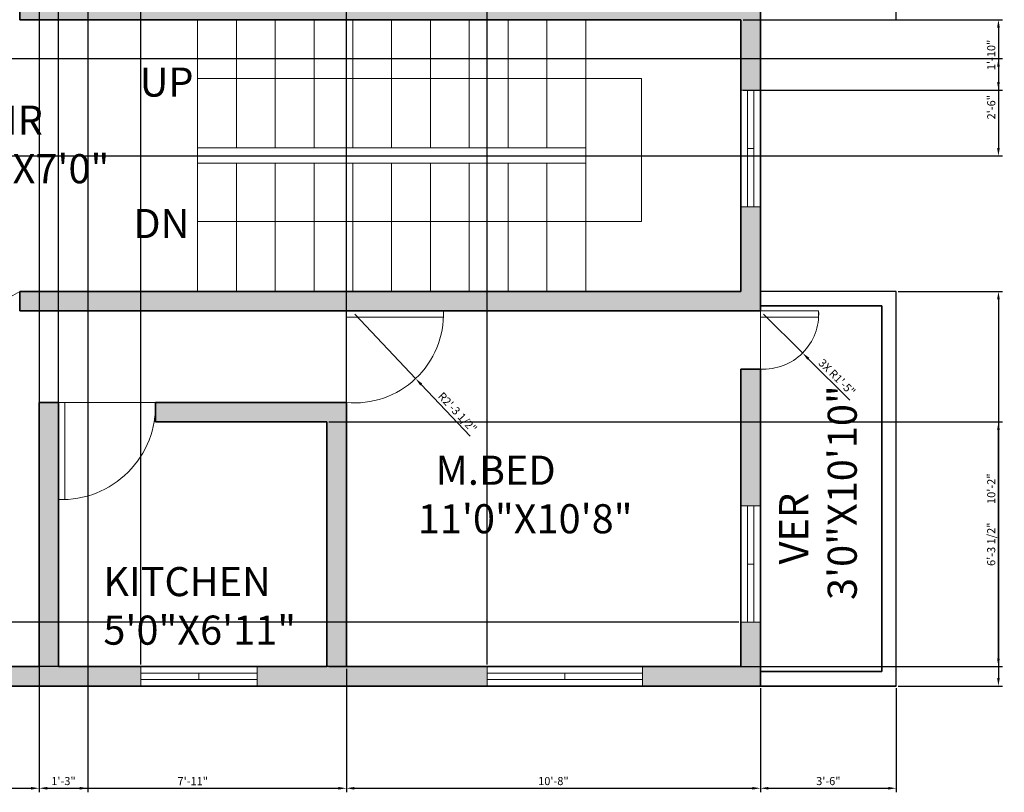
# Model space of a CAD drawing. Units: inches. Extents: x 5145 to 5807, y 9597 to 10060.
# Tile 2 of 3: x 5502 to 5807, y 9597 to 9836. Entities that reach past the tile are written whole.
import ezdxf

# ---------------------------------------------------------------- set-up
doc = ezdxf.new("R2010")
doc.units = ezdxf.units.IN
for name, color, linetype, lineweight in [('A-ANNO-DIMS', 7, 'Continuous', 18), ('A-AREA-IDEN', 7, 'Continuous', 18), ('A-GLAZ', 140, 'Continuous', 18), ('A-WALL', 7, 'Continuous', 35)]:
    doc.layers.add(name, color=color, linetype=linetype, lineweight=lineweight)
for name, color, linetype, lineweight, true_color in [('A-ANNO-SYMB', 244, 'Continuous', 18, 0x991b1e), ('A-ANNO-TEXT', 244, 'Continuous', 18, 0x991b1e), ('A-DOOR', 2, 'Continuous', 18, 0xf1eb1f), ('A-FLOR-STRS', 30, 'Continuous', 18, 0xf26722), ('A-WALL-PATT', 159, 'Continuous', 13, 0x22346e), ('A-WALL-PRPT', 61, 'Continuous', 25, 0xedee99)]:
    doc.layers.add(name, color=color, linetype=linetype, lineweight=lineweight, true_color=true_color)
doc.styles.get("Standard").update_dxf_attribs({"font": 'arial.ttf'})
doc.dimstyles.new('ISO-25', dxfattribs={"dimtxt": 2.5, "dimasz": 2.5, "dimexe": 1.25, "dimexo": 0.625, "dimtad": 1, "dimlunit": 3, "dimtxsty": 'Standard', "dimcen": 2.5, "dimadec": 0, "dimazin": 0, "dimtfac": 1, "dimtmove": 0, "dimatfit": 3, "dimfxl": 1, "dimarcsym": 0})

# ---------------------------------------------------------------- blocks, each defined once
blk = doc.blocks.new('WIN-36IN')
for p, q in [((0, 6), (0, 0)), ((0, 6), (36, 6)), ((0, 4), (36, 4)), ((18, 2), (18, 4)), ((36, 0), (36, 6)), ((0, 2), (36, 2)), ((36, 0), (0, 0))]:
    blk.add_line(p, q)
blk = doc.blocks.new('WIN-48IN')
for p, q in [((6, 48), (0, 48)), ((0, 48), (0, 0)), ((2, 0), (2, 48)), ((4, 0), (4, 48)), ((6, 0), (6, 48)), ((4, 24), (2, 24)), ((0, 0), (6, 0))]:
    blk.add_line(p, q)
blk = doc.blocks.new('DOOR-SWING-18IN')
for p, q in [((0.03, 18.03), (18.03, 18.03)), ((16.03, 0.03), (16.03, 18.03)), ((16.03, 18.03), (18.03, 18.03)), ((18.03, 18.03), (18.03, 0.03)), ((18.03, 0.03), (16.03, 0.03))]:
    blk.add_line(p, q)
blk.add_arc((17.03, 17.03), 17.03, 176.6335, 273.3665)
blk = doc.blocks.new('DOOR-SWING-30IN')
for p, q in [((0, 0), (0, 30)), ((0, 30), (2, 30)), ((2, 30), (2, 0)), ((2, 0), (0, 0)), ((0, 0), (30, 0))]:
    blk.add_line(p, q)
blk.add_arc((1, 1), 29.02, 358.0251, 91.9749)
blk = doc.blocks.new('*D23')
at = {"layer": 'A-ANNO-DIMS', "color": 0, "lineweight": -2, "transparency": 16777216}
for p, q in [((5329.12, 9635.64), (5329.12, 9597.42)), ((5508.12, 9635.64), (5508.12, 9597.42)), ((5331.62, 9598.67), (5505.62, 9598.67))]:
    blk.add_line(p, q, dxfattribs=at)
at = {"layer": 'A-ANNO-DIMS', "color": 0, "transparency": 16777216}
for points in [[(5331.62, 9599.08), (5331.62, 9598.25), (5329.12, 9598.67)], [(5505.62, 9599.08), (5505.62, 9598.25), (5508.12, 9598.67)]]:
    blk.add_solid(points, dxfattribs=at)
at = {"layer": 'Defpoints', "color": 0, "transparency": 16777216}
for p in [(5329.12, 9636.27), (5508.12, 9636.27), (5508.12, 9598.67)]:
    blk.add_point(p, dxfattribs=at)
at = {"layer": 'A-ANNO-DIMS', "color": 0, "transparency": 16777216, "insert": (5418.62, 9600.55), "char_height": 2.5, "attachment_point": 5}
blk.add_mtext('14\'-11"', dxfattribs=at)
blk = doc.blocks.new('*D24')
at = {"layer": 'A-ANNO-DIMS', "color": 0, "lineweight": -2, "transparency": 16777216}
for p, q in [((5508.12, 9635.64), (5508.12, 9597.42)), ((5603.12, 9635.64), (5603.12, 9597.42)), ((5510.62, 9598.67), (5600.62, 9598.67))]:
    blk.add_line(p, q, dxfattribs=at)
at = {"layer": 'A-ANNO-DIMS', "color": 0, "transparency": 16777216}
for points in [[(5510.62, 9599.08), (5510.62, 9598.25), (5508.12, 9598.67)], [(5600.62, 9599.08), (5600.62, 9598.25), (5603.12, 9598.67)]]:
    blk.add_solid(points, dxfattribs=at)
at = {"layer": 'Defpoints', "color": 0, "transparency": 16777216}
for p in [(5508.12, 9636.27), (5603.12, 9636.27), (5603.12, 9598.67)]:
    blk.add_point(p, dxfattribs=at)
at = {"layer": 'A-ANNO-DIMS', "color": 0, "transparency": 16777216, "insert": (5555.62, 9600.55), "char_height": 2.5, "attachment_point": 5}
blk.add_mtext('7\'-11"', dxfattribs=at)
blk = doc.blocks.new('*D25')
at = {"layer": 'A-ANNO-DIMS', "color": 0, "lineweight": -2, "transparency": 16777216}
for p, q in [((5603.12, 9635.64), (5603.12, 9597.42)), ((5731.12, 9629.64), (5731.12, 9597.42)), ((5605.62, 9598.67), (5728.62, 9598.67))]:
    blk.add_line(p, q, dxfattribs=at)
at = {"layer": 'A-ANNO-DIMS', "color": 0, "transparency": 16777216}
for points in [[(5605.62, 9599.08), (5605.62, 9598.25), (5603.12, 9598.67)], [(5728.62, 9599.08), (5728.62, 9598.25), (5731.12, 9598.67)]]:
    blk.add_solid(points, dxfattribs=at)
at = {"layer": 'Defpoints', "color": 0, "transparency": 16777216}
for p in [(5603.12, 9636.27), (5731.12, 9630.27), (5731.12, 9598.67)]:
    blk.add_point(p, dxfattribs=at)
at = {"layer": 'A-ANNO-DIMS', "color": 0, "transparency": 16777216, "insert": (5667.12, 9600.57), "char_height": 2.5, "attachment_point": 5}
blk.add_mtext('10\'-8"', dxfattribs=at)
blk = doc.blocks.new('*D26')
at = {"layer": 'A-ANNO-DIMS', "color": 0, "lineweight": -2, "transparency": 16777216}
for p, q in [((5731.12, 9629.64), (5731.12, 9597.42)), ((5773.12, 9629.64), (5773.12, 9597.42)), ((5733.62, 9598.67), (5770.62, 9598.67))]:
    blk.add_line(p, q, dxfattribs=at)
at = {"layer": 'A-ANNO-DIMS', "color": 0, "transparency": 16777216}
for points in [[(5733.62, 9599.08), (5733.62, 9598.25), (5731.12, 9598.67)], [(5770.62, 9599.08), (5770.62, 9598.25), (5773.12, 9598.67)]]:
    blk.add_solid(points, dxfattribs=at)
at = {"layer": 'Defpoints', "color": 0, "transparency": 16777216}
for p in [(5731.12, 9630.27), (5773.12, 9630.27), (5773.12, 9598.67)]:
    blk.add_point(p, dxfattribs=at)
at = {"layer": 'A-ANNO-DIMS', "color": 0, "transparency": 16777216, "insert": (5752.12, 9600.57), "char_height": 2.5, "attachment_point": 5}
blk.add_mtext('3\'-6"', dxfattribs=at)
blk = doc.blocks.new('*D28')
at = {"layer": 'A-ANNO-DIMS', "color": 0, "lineweight": -2, "transparency": 16777216}
for p, q in [((5773.74, 9752.27), (5805.97, 9752.27)), ((5804.72, 9749.77), (5804.72, 9632.77)), ((5773.74, 9630.27), (5805.97, 9630.27))]:
    blk.add_line(p, q, dxfattribs=at)
at = {"layer": 'A-ANNO-DIMS', "color": 0, "transparency": 16777216}
for points in [[(5804.3, 9749.77), (5805.13, 9749.77), (5804.72, 9752.27)], [(5804.3, 9632.77), (5805.13, 9632.77), (5804.72, 9630.27)]]:
    blk.add_solid(points, dxfattribs=at)
at = {"layer": 'Defpoints', "color": 0, "transparency": 16777216}
for p in [(5773.12, 9752.27), (5773.12, 9630.27), (5804.72, 9630.27)]:
    blk.add_point(p, dxfattribs=at)
at = {"layer": 'A-ANNO-DIMS', "color": 0, "transparency": 16777216, "insert": (5802.81, 9691.27), "char_height": 2.5, "attachment_point": 5, "rotation": 90}
blk.add_mtext('10\'-2"', dxfattribs=at)
blk = doc.blocks.new('*D30')
at = {"layer": 'A-ANNO-DIMS', "color": 0, "lineweight": -2, "transparency": 16777216}
for p, q in [((5597.74, 9711.93), (5805.97, 9711.93)), ((5804.72, 9638.77), (5804.72, 9709.43)), ((5597.74, 9636.27), (5805.97, 9636.27))]:
    blk.add_line(p, q, dxfattribs=at)
at = {"layer": 'A-ANNO-DIMS', "color": 0, "transparency": 16777216}
for points in [[(5804.3, 9709.43), (5805.13, 9709.43), (5804.72, 9711.93)], [(5804.3, 9638.77), (5805.13, 9638.77), (5804.72, 9636.27)]]:
    blk.add_solid(points, dxfattribs=at)
at = {"layer": 'Defpoints', "color": 0, "transparency": 16777216}
for p in [(5597.12, 9711.93), (5804.72, 9711.93), (5597.12, 9636.27)]:
    blk.add_point(p, dxfattribs=at)
at = {"layer": 'A-ANNO-DIMS', "color": 0, "transparency": 16777216, "insert": (5802.8, 9674.1), "char_height": 2.5, "attachment_point": 5, "rotation": 90}
blk.add_mtext('6\'-3 1/2"', dxfattribs=at)
blk = doc.blocks.new('*D37')
at = {"layer": 'A-ANNO-DIMS', "color": 0, "lineweight": -2, "transparency": 16777216}
for p, q in [((5508.12, 10015.64), (5508.12, 9597.42)), ((5523.2, 10015.64), (5523.2, 9597.42)), ((5510.62, 9598.67), (5520.7, 9598.67))]:
    blk.add_line(p, q, dxfattribs=at)
at = {"layer": 'A-ANNO-DIMS', "color": 0, "transparency": 16777216}
for points in [[(5510.62, 9599.08), (5510.62, 9598.25), (5508.12, 9598.67)], [(5520.7, 9599.08), (5520.7, 9598.25), (5523.2, 9598.67)]]:
    blk.add_solid(points, dxfattribs=at)
at = {"layer": 'Defpoints', "color": 0, "transparency": 16777216}
for p in [(5508.12, 10016.27), (5523.2, 10016.27), (5523.2, 9598.67)]:
    blk.add_point(p, dxfattribs=at)
at = {"layer": 'A-ANNO-DIMS', "color": 0, "transparency": 16777216, "insert": (5515.66, 9600.57), "char_height": 2.5, "attachment_point": 5}
blk.add_mtext('1\'-3"', dxfattribs=at)
blk = doc.blocks.new('*D43')
at = {"layer": 'A-ANNO-DIMS', "color": 0, "lineweight": -2, "transparency": 16777216}
for p, q in [((5514.12, 9636.89), (5514.12, 10055.12)), ((5539.54, 9636.89), (5539.54, 10055.12)), ((5516.62, 10053.87), (5537.04, 10053.87))]:
    blk.add_line(p, q, dxfattribs=at)
at = {"layer": 'A-ANNO-DIMS', "color": 0, "transparency": 16777216}
for points in [[(5516.62, 10054.28), (5516.62, 10053.45), (5514.12, 10053.87)], [(5537.04, 10054.28), (5537.04, 10053.45), (5539.54, 10053.87)]]:
    blk.add_solid(points, dxfattribs=at)
at = {"layer": 'Defpoints', "color": 0, "transparency": 16777216}
for p in [(5539.54, 10053.87), (5514.12, 9636.27), (5539.54, 9636.27)]:
    blk.add_point(p, dxfattribs=at)
at = {"layer": 'A-ANNO-DIMS', "color": 0, "transparency": 16777216, "insert": (5526.83, 10055.79), "char_height": 2.5, "attachment_point": 5}
blk.add_mtext('2\'-1 1/2"', dxfattribs=at)
blk = doc.blocks.new('*D44')
at = {"layer": 'A-ANNO-DIMS', "color": 0, "lineweight": -2, "transparency": 16777216}
for p, q in [((5603.12, 9636.89), (5603.12, 10055.12)), ((5646.69, 9636.89), (5646.69, 10055.12)), ((5605.62, 10053.87), (5644.19, 10053.87))]:
    blk.add_line(p, q, dxfattribs=at)
at = {"layer": 'A-ANNO-DIMS', "color": 0, "transparency": 16777216}
for points in [[(5605.62, 10054.28), (5605.62, 10053.45), (5603.12, 10053.87)], [(5644.19, 10054.28), (5644.19, 10053.45), (5646.69, 10053.87)]]:
    blk.add_solid(points, dxfattribs=at)
at = {"layer": 'Defpoints', "color": 0, "transparency": 16777216}
for p in [(5646.69, 10053.87), (5603.12, 9636.27), (5646.69, 9636.27)]:
    blk.add_point(p, dxfattribs=at)
at = {"layer": 'A-ANNO-DIMS', "color": 0, "transparency": 16777216, "insert": (5624.91, 10055.79), "char_height": 2.5, "attachment_point": 5}
blk.add_mtext('3\'-7 1/2"', dxfattribs=at)
blk = doc.blocks.new('*D46')
at = {"layer": 'A-ANNO-DIMS', "color": 0, "lineweight": -2, "transparency": 16777216}
for p, q in [((5188.74, 9824.27), (5805.97, 9824.27)), ((5804.72, 9821.77), (5804.72, 9796.64)), ((5188.74, 9794.14), (5805.97, 9794.14))]:
    blk.add_line(p, q, dxfattribs=at)
at = {"layer": 'A-ANNO-DIMS', "color": 0, "transparency": 16777216}
for points in [[(5804.3, 9821.77), (5805.13, 9821.77), (5804.72, 9824.27)], [(5804.3, 9796.64), (5805.13, 9796.64), (5804.72, 9794.14)]]:
    blk.add_solid(points, dxfattribs=at)
at = {"layer": 'Defpoints', "color": 0, "transparency": 16777216}
for p in [(5188.12, 9824.27), (5188.12, 9794.14), (5804.72, 9794.14)]:
    blk.add_point(p, dxfattribs=at)
at = {"layer": 'A-ANNO-DIMS', "color": 0, "transparency": 16777216, "insert": (5802.81, 9809.2), "char_height": 2.5, "attachment_point": 5, "rotation": 90}
blk.add_mtext('2\'-6"', dxfattribs=at)
blk = doc.blocks.new('*D48')
at = {"layer": 'A-ANNO-DIMS', "color": 0, "lineweight": -2, "transparency": 16777216}
for p, q in [((5725.74, 9836.27), (5805.97, 9836.27)), ((5804.72, 9833.77), (5804.72, 9816.96)), ((5725.74, 9814.46), (5805.97, 9814.46))]:
    blk.add_line(p, q, dxfattribs=at)
at = {"layer": 'A-ANNO-DIMS', "color": 0, "transparency": 16777216}
for points in [[(5804.3, 9833.77), (5805.13, 9833.77), (5804.72, 9836.27)], [(5804.3, 9816.96), (5805.13, 9816.96), (5804.72, 9814.46)]]:
    blk.add_solid(points, dxfattribs=at)
at = {"layer": 'Defpoints', "color": 0, "transparency": 16777216}
for p in [(5725.12, 9836.27), (5725.12, 9814.46), (5804.72, 9814.46)]:
    blk.add_point(p, dxfattribs=at)
at = {"layer": 'A-ANNO-DIMS', "color": 0, "transparency": 16777216, "insert": (5802.81, 9825.36), "char_height": 2.5, "attachment_point": 5, "rotation": 90}
blk.add_mtext('1\'-10"', dxfattribs=at)
blk = doc.blocks.new('*D49')
at = {"layer": 'A-ANNO-DIMS', "color": 0, "lineweight": -2, "transparency": 16777216}
for p, q in [((5724.49, 9649.99), (5149.27, 9649.99)), ((5150.52, 9638.77), (5150.52, 9647.49)), ((5724.49, 9636.27), (5149.27, 9636.27))]:
    blk.add_line(p, q, dxfattribs=at)
at = {"layer": 'A-ANNO-DIMS', "color": 0, "transparency": 16777216}
for points in [[(5150.1, 9647.49), (5150.93, 9647.49), (5150.52, 9649.99)], [(5150.1, 9638.77), (5150.93, 9638.77), (5150.52, 9636.27)]]:
    blk.add_solid(points, dxfattribs=at)
at = {"layer": 'Defpoints', "color": 0, "transparency": 16777216}
for p in [(5150.52, 9649.99), (5725.12, 9649.99), (5725.12, 9636.27)]:
    blk.add_point(p, dxfattribs=at)
at = {"layer": 'A-ANNO-DIMS', "color": 0, "transparency": 16777216, "insert": (5148.6, 9643.13), "char_height": 2.5, "attachment_point": 5, "rotation": 90}
blk.add_mtext('1\'-1 1/2"', dxfattribs=at)
blk = doc.blocks.new('*D55')
at = {"layer": 'A-ANNO-DIMS', "color": 0, "lineweight": -2, "transparency": 16777216}
for p, q in [((5605.68, 9745.27), (5624.53, 9725.31)), ((5641.38, 9707.47), (5626.25, 9723.49))]:
    blk.add_line(p, q, dxfattribs=at)
at = {"layer": 'A-ANNO-DIMS', "color": 0, "transparency": 16777216}
blk.add_solid([(5626.55, 9723.78), (5625.95, 9723.2), (5624.53, 9725.31)], dxfattribs=at)
at = {"layer": 'Defpoints', "color": 0, "transparency": 16777216}
for p in [(5605.68, 9745.27), (5624.53, 9725.31)]:
    blk.add_point(p, dxfattribs=at)
at = {"layer": 'A-ANNO-DIMS', "color": 0, "transparency": 16777216, "insert": (5637.24, 9714.65), "char_height": 2.5, "attachment_point": 5, "rotation": 313.3682}
blk.add_mtext('R2\'-3 1/2"', dxfattribs=at)
blk = doc.blocks.new('*D58')
at = {"layer": 'A-ANNO-DIMS', "color": 0, "lineweight": -2, "transparency": 16777216}
for p, q in [((5732.12, 9745.27), (5744.16, 9733.23)), ((5758.77, 9718.62), (5745.93, 9731.46))]:
    blk.add_line(p, q, dxfattribs=at)
at = {"layer": 'A-ANNO-DIMS', "color": 0, "transparency": 16777216}
blk.add_solid([(5746.22, 9731.75), (5745.63, 9731.16), (5744.16, 9733.23)], dxfattribs=at)
at = {"layer": 'Defpoints', "color": 0, "transparency": 16777216}
for p in [(5732.12, 9745.27), (5744.16, 9733.23)]:
    blk.add_point(p, dxfattribs=at)
at = {"layer": 'A-ANNO-DIMS', "color": 0, "transparency": 16777216, "insert": (5754.57, 9725.5), "char_height": 2.5, "attachment_point": 5, "rotation": 315.0004}
blk.add_mtext('3X R1\'-5"', dxfattribs=at)

msp = doc.modelspace()

# ---------------------------------------------------------------- hatches: boundary and pattern name
at = {"layer": 'A-WALL-PATT'}
h = msp.add_hatch(color=256, dxfattribs=at)
h.dxf.hatch_style = 1
h.paths.add_polyline_path([(5244.116, 10016.267), (5266.307, 10016.267), (5266.307, 10022.267), (5238.116, 10022.267), (5238.116, 10017.767), (5238.116, 9962.267), (5329.116, 9962.267), (5329.116, 9968.267), (5311.116, 9968.267), (5244.116, 9968.267)])
h.paths.add_polyline_path([(5372.995, 10022.267), (5290.307, 10022.267), (5290.307, 10016.267), (5323.116, 10016.267), (5323.116, 9986.267), (5327.116, 9986.267, -0.0293864), (5329.116, 9986.267), (5329.116, 10016.267), (5372.995, 10016.267)])
h.paths.add_polyline_path([(5523.196, 10022.267), (5432.995, 10022.267), (5432.995, 10016.267), (5502.116, 10016.267), (5502.116, 9878.267), (5508.116, 9878.267), (5508.116, 9908.267), (5508.116, 10016.267), (5523.196, 10016.267)])
h.paths.add_polyline_path([(5623.247, 10022.267), (5559.196, 10022.267), (5559.196, 10016.267), (5591.116, 10016.267), (5591.116, 9884.267), (5538.116, 9884.267), (5538.116, 9880.267, -0.0172363), (5538.116, 9878.267), (5597.116, 9878.267), (5597.116, 10016.267), (5623.247, 10016.267)])
h.paths.add_polyline_path([(5731.116, 10022.267), (5695.247, 10022.267), (5695.247, 10016.267), (5725.116, 10016.267), (5725.116, 9968.267), (5731.116, 9968.267)])
h.paths.add_polyline_path([(5731.116, 9920.267), (5725.116, 9920.267), (5725.116, 9860.267, -0.0293864), (5727.116, 9860.267), (5731.116, 9860.267)])
h.paths.add_polyline_path([(5731.116, 9842.267), (5725.116, 9842.267), (5502.116, 9842.267), (5502.116, 9836.267), (5725.116, 9836.267), (5725.116, 9814.459), (5731.116, 9814.459)])
h.paths.add_polyline_path([(5731.116, 9778.459), (5725.116, 9778.459), (5725.116, 9752.267), (5502.116, 9752.267), (5502.116, 9746.267), (5731.116, 9746.267)])
h.paths.add_polyline_path([(5514.116, 9717.93), (5508.116, 9717.93), (5508.116, 9704.267), (5508.116, 9636.267), (5460.439, 9636.267), (5460.439, 9630.267), (5539.543, 9630.267), (5539.543, 9636.267), (5514.116, 9636.267), (5514.116, 9704.267)])
h.paths.add_polyline_path([(5603.116, 9717.93), (5544.116, 9717.93, -0.0172363), (5544.116, 9715.93), (5544.116, 9711.93), (5597.116, 9711.93), (5597.116, 9636.267), (5575.543, 9636.267), (5575.543, 9630.267), (5646.695, 9630.267), (5646.695, 9636.267), (5603.116, 9636.267), (5603.116, 9704.267)])
h.paths.add_polyline_path([(5731.116, 9649.987), (5725.116, 9649.987), (5725.116, 9636.267), (5694.695, 9636.267), (5694.695, 9630.267), (5731.116, 9630.267)])
h.paths.add_polyline_path([(5731.116, 9728.267), (5725.116, 9728.267), (5725.116, 9685.987), (5731.116, 9685.987)])
h.paths.add_polyline_path([(5400.439, 9636.267), (5329.116, 9636.267), (5329.116, 9662.267, -0.0217289), (5327.116, 9662.267), (5323.116, 9662.267), (5323.116, 9636.267), (5283.616, 9636.267), (5283.616, 9630.267), (5329.116, 9630.267), (5400.439, 9630.267)])
h.paths.add_polyline_path([(5263.165, 9636.267), (5244.116, 9636.267), (5244.116, 9686.267), (5329.116, 9686.267), (5329.116, 9692.267), (5287.116, 9692.267), (5238.116, 9692.267), (5238.116, 9674.267), (5238.116, 9630.267), (5263.165, 9630.267)])
h.paths.add_polyline_path([(5220.116, 9690.267, -0.0293864), (5220.116, 9692.267), (5188.116, 9692.267), (5188.116, 9734.135), (5182.116, 9734.135), (5182.116, 9686.267), (5220.116, 9686.267)])
h.paths.add_polyline_path([(5329.116, 9794.267), (5469.593, 9794.267), (5469.593, 9800.267), (5427.593, 9800.267), (5329.116, 9800.267), (5329.116, 9830.267), (5329.116, 9920.267, -0.0121933), (5327.116, 9920.267), (5323.116, 9920.267), (5323.116, 9830.267), (5188.116, 9830.267), (5188.116, 9865.614), (5182.116, 9865.614), (5182.116, 9794.135), (5188.116, 9794.135), (5188.116, 9824.267), (5323.116, 9824.267), (5323.116, 9734.267), (5327.116, 9734.267, -0.0121933), (5329.116, 9734.267)])

# ---------------------------------------------------------------- linework, layer by layer
at = {"layer": 'A-ANNO-SYMB'}
for p, q in [((5694.376, 9818.125), (5557.116, 9818.125)), ((5694.376, 9773.836), (5694.376, 9818.125)), ((5557.116, 9773.836), (5694.376, 9773.836))]:
    msp.add_line(p, q, dxfattribs=at)
at = {"layer": 'A-DOOR'}
for p, q in [((5603.116, 9746.267), (5633.116, 9746.267)), ((5603.116, 9744.267), (5603.116, 9746.267)), ((5603.116, 9717.93), (5603.116, 9746.267)), ((5633.116, 9744.267), (5603.116, 9744.267)), ((5633.116, 9746.267), (5633.116, 9744.267))]:
    msp.add_line(p, q, dxfattribs=at)
for centre, radius, start, end in [((5476.126, 9793.267), 48.544, 178.81962, 302.37097), ((5605.677, 9745.267), 27.457, 264.64826, 2.08719)]:
    msp.add_arc(centre, radius, start, end, dxfattribs=at)
at = {"layer": 'A-FLOR-STRS'}
for p, q in [((5557.116, 9836.267), (5557.116, 9752.267)), ((5569.116, 9836.267), (5569.116, 9796.667)), ((5581.116, 9836.267), (5581.116, 9796.667)), ((5593.116, 9836.267), (5593.116, 9796.667)), ((5605.116, 9836.267), (5605.116, 9796.667)), ((5617.116, 9836.267), (5617.116, 9796.667)), ((5629.116, 9836.267), (5629.116, 9796.667)), ((5641.116, 9836.267), (5641.116, 9796.667)), ((5653.116, 9836.267), (5653.116, 9796.667)), ((5665.116, 9836.267), (5665.116, 9796.667)), ((5677.116, 9752.267), (5677.116, 9836.267)), ((5677.116, 9836.267), (5677.116, 9752.267)), ((5557.116, 9796.667), (5677.116, 9796.667)), ((5557.116, 9796.667), (5677.116, 9796.667)), ((5557.116, 9791.867), (5677.116, 9791.867)), ((5557.116, 9791.867), (5677.116, 9791.867)), ((5569.116, 9791.867), (5569.116, 9752.267)), ((5581.116, 9791.867), (5581.116, 9752.267)), ((5593.116, 9791.867), (5593.116, 9752.267)), ((5605.116, 9791.867), (5605.116, 9752.267)), ((5617.116, 9791.867), (5617.116, 9752.267)), ((5629.116, 9791.867), (5629.116, 9752.267)), ((5641.116, 9791.867), (5641.116, 9752.267)), ((5653.116, 9791.867), (5653.116, 9752.267)), ((5665.116, 9791.867), (5665.116, 9752.267))]:
    msp.add_line(p, q, dxfattribs=at)
at = {"layer": 'A-GLAZ'}
for p, q in [((5725.116, 9814.459), (5731.116, 9814.459)), ((5731.116, 9778.459), (5731.116, 9814.459)), ((5731.116, 9778.459), (5725.116, 9778.459)), ((5725.116, 9685.987), (5731.116, 9685.987)), ((5731.116, 9649.987), (5731.116, 9685.987)), ((5725.116, 9649.987), (5731.116, 9649.987)), ((5539.543, 9630.267), (5539.543, 9636.267)), ((5575.543, 9636.267), (5575.543, 9630.267)), ((5646.695, 9630.267), (5646.695, 9636.267)), ((5694.695, 9636.267), (5694.695, 9630.267)), ((5539.543, 9630.267), (5575.543, 9630.267)), ((5646.695, 9630.267), (5694.695, 9630.267))]:
    msp.add_line(p, q, dxfattribs=at)
at = {"layer": 'A-WALL'}
for p, q in [((5502.116, 9842.267), (5502.116, 9836.267)), ((5731.116, 9746.267), (5731.116, 9842.267)), ((5502.116, 9836.267), (5725.116, 9836.267)), ((5725.116, 9752.267), (5725.116, 9836.267)), ((5502.116, 9752.267), (5725.116, 9752.267)), ((5502.116, 9752.267), (5502.116, 9746.267)), ((5502.116, 9746.267), (5731.116, 9746.267)), ((5725.116, 9636.267), (5725.116, 9728.267)), ((5725.116, 9728.267), (5731.116, 9728.267)), ((5731.116, 9630.267), (5731.116, 9728.267)), ((5514.116, 9717.93), (5508.116, 9717.93)), ((5508.116, 9717.93), (5508.116, 9704.267)), ((5514.116, 9704.267), (5514.116, 9717.93)), ((5603.116, 9717.93), (5544.116, 9717.93)), ((5544.116, 9711.93), (5544.116, 9717.93)), ((5603.116, 9717.93), (5603.116, 9704.267)), ((5603.116, 9704.267), (5603.116, 9717.93)), ((5597.116, 9711.93), (5544.116, 9711.93)), ((5597.116, 9636.267), (5597.116, 9711.93)), ((5508.116, 9636.267), (5508.116, 9704.267)), ((5514.116, 9636.267), (5514.116, 9704.267)), ((5603.116, 9636.267), (5603.116, 9704.267)), ((5329.116, 9636.267), (5508.116, 9636.267)), ((5514.116, 9636.267), (5597.116, 9636.267)), ((5603.116, 9636.267), (5725.116, 9636.267)), ((5329.116, 9630.267), (5773.116, 9630.267))]:
    msp.add_line(p, q, dxfattribs=at)
at = {"layer": 'A-WALL-PRPT'}
for p, q in [((5773.116, 9836.267), (5773.116, 10022.267)), ((5773.116, 9836.267), (5773.116, 9878.267)), ((5731.116, 9836.267), (5773.116, 9836.267)), ((5731.116, 9836.267), (5773.116, 9836.267)), ((5773.116, 9752.267), (5731.116, 9752.267)), ((5773.116, 9752.267), (5731.116, 9752.267)), ((5773.116, 9746.267), (5773.116, 9752.267)), ((5773.116, 9630.267), (5773.116, 9752.267)), ((5768.616, 9747.767), (5731.116, 9747.767)), ((5731.116, 9747.767), (5768.616, 9747.767)), ((5768.616, 9662.267), (5768.616, 9747.767)), ((5768.616, 9747.767), (5768.616, 9634.767)), ((5773.116, 9662.267), (5773.116, 9746.267)), ((5768.616, 9634.767), (5768.616, 9662.267)), ((5773.116, 9630.267), (5773.116, 9662.267)), ((5731.116, 9634.767), (5768.616, 9634.767)), ((5768.616, 9634.767), (5731.116, 9634.767)), ((5731.116, 9630.267), (5773.116, 9630.267))]:
    msp.add_line(p, q, dxfattribs=at)

# ---------------------------------------------------------------- block references
at = {"layer": 'A-DOOR', "rotation": 90.00000000001049}
msp.add_blockref('DOOR-SWING-18IN', (5749.146, 9728.238), dxfattribs=at)
at = {"layer": 'A-DOOR', "extrusion": (0, 0, -1), "zscale": -1, "rotation": 180}
msp.add_blockref('DOOR-SWING-30IN', (-5514.116, 9717.93), dxfattribs=at)
at = {"layer": 'A-GLAZ'}
for name, p, rotation in [('WIN-36IN', (5725.116, 9814.459), 270.0000000000075), ('WIN-36IN', (5725.116, 9685.987), 270.0000000000065), ('WIN-36IN', (5575.543, 9636.268), 180), ('WIN-48IN', (5646.694, 9636.268), 270.0000000000176)]:
    msp.add_blockref(name, p, dxfattribs=dict(at, rotation=rotation))

# ---------------------------------------------------------------- texts
at = {"layer": 'A-ANNO-TEXT', "char_height": 9, "attachment_point": 1}
for s, width, heights, insert in [('{UP}', 8.14646, [0], (5539.229, 9821.487)), ('{ DN}', 23.17085, [16.878], (5534.491, 9777.76))]:
    msp.add_mtext_dynamic_manual_height_columns(s, width=width, gutter_width=12.5, heights=heights, dxfattribs=dict(at, insert=insert))
at = {"layer": 'A-AREA-IDEN', "char_height": 9, "attachment_point": 1}
for s, width, heights, insert in [('  STAIR\\P16\'5"X7\'0"', 91.95952, [57.275], (5470.253, 9809.7)), ('  M.BED\\P11\'0"X10\'8"', 51.95741, [0], (5625.199, 9701.489)), (' KITCHEN\\P 5\'0"X6\'11"', 76.31305, [51.205], (5525.234, 9667.054))]:
    msp.add_mtext_dynamic_manual_height_columns(s, width=width, gutter_width=12.5, heights=heights, dxfattribs=dict(at, insert=insert))
at = {"layer": 'A-AREA-IDEN', "insert": (5736.916, 9656.871), "char_height": 9, "attachment_point": 1, "rotation": 90}
msp.add_mtext_dynamic_manual_height_columns('    VER\\P3\'0"X10\'10"', width=68.70978, gutter_width=12.5, heights=[37.922], dxfattribs=at)

# ---------------------------------------------------------------- dimensions: what is measured, and where the dimension line sits
at = {"layer": 'A-ANNO-DIMS'}
for base, p1, p2, picture, middle in [((5539.543, 10053.867), (5514.116, 9636.267), (5539.543, 9636.267), '*D43', (5526.83, 10055.785)), ((5646.695, 10053.867), (5603.116, 9636.267), (5646.695, 9636.267), '*D44', (5624.906, 10055.786)), ((5523.196, 9598.667), (5508.116, 10016.267), (5523.196, 10016.267), '*D37', (5515.656, 9600.57)), ((5508.116, 9598.667), (5329.116, 9636.267), (5508.116, 9636.267), '*D23', (5418.616, 9600.548)), ((5603.116, 9598.667), (5508.116, 9636.267), (5603.116, 9636.267), '*D24', (5555.616, 9600.548)), ((5731.116, 9598.667), (5603.116, 9636.267), (5731.116, 9630.267), '*D25', (5667.116, 9600.569)), ((5773.116, 9598.667), (5731.116, 9630.267), (5773.116, 9630.267), '*D26', (5752.116, 9600.57))]:
    dim = msp.add_linear_dim(base=base, p1=p1, p2=p2, dimstyle='ISO-25', override={"dimdec": 1, "dimlfac": 1, "dimrnd": 0, "dimzin": 1, "dimdsep": 46, "dimlunit": 4, "dimfrac": 2}, dxfattribs=at)
    dim.commit()
    dim.dimension.update_dxf_attribs({"geometry": picture, "text_midpoint": middle})
for base, p1, p2, picture, middle in [((5804.716, 9814.459), (5725.116, 9836.267), (5725.116, 9814.459), '*D48', (5802.815, 9825.363)), ((5804.716, 9794.135), (5188.116, 9824.267), (5188.116, 9794.135), '*D46', (5802.815, 9809.201)), ((5804.716, 9630.267), (5773.116, 9752.267), (5773.116, 9630.267), '*D28', (5802.815, 9691.267)), ((5804.716, 9711.93), (5597.116, 9636.267), (5597.116, 9711.93), '*D30', (5802.798, 9674.099)), ((5150.516, 9649.987), (5725.116, 9636.267), (5725.116, 9649.987), '*D49', (5148.599, 9643.127))]:
    dim = msp.add_linear_dim(base=base, p1=p1, p2=p2, angle=90, dimstyle='ISO-25', override={"dimdec": 1, "dimlfac": 1, "dimrnd": 0, "dimzin": 1, "dimdsep": 46, "dimlunit": 4, "dimfrac": 2}, dxfattribs=at)
    dim.commit()
    dim.dimension.update_dxf_attribs({"geometry": picture, "text_midpoint": middle})
dim = msp.add_radius_dim(center=(5605.677, 9745.267), mpoint=(5624.532, 9725.307), dimstyle='ISO-25', override={"dimdec": 1, "dimlfac": 1, "dimrnd": 0, "dimzin": 1, "dimdsep": 46, "dimlunit": 4, "dimfrac": 2}, dxfattribs=at)
dim.commit()
dim.dimension.update_dxf_attribs({"geometry": '*D55', "text_midpoint": (5635.845, 9713.331), "dimtype": 164})
dim = msp.add_radius_dim(center=(5732.116, 9745.267), mpoint=(5744.158, 9733.226), text='3X <>', dimstyle='ISO-25', override={"dimdec": 1, "dimlfac": 1, "dimrnd": 0, "dimzin": 1, "dimdsep": 46, "dimlunit": 4, "dimfrac": 2}, dxfattribs=at)
dim.commit()
dim.dimension.update_dxf_attribs({"geometry": '*D58', "text_midpoint": (5754.575, 9725.5)})

doc.saveas('drawing.dxf')
